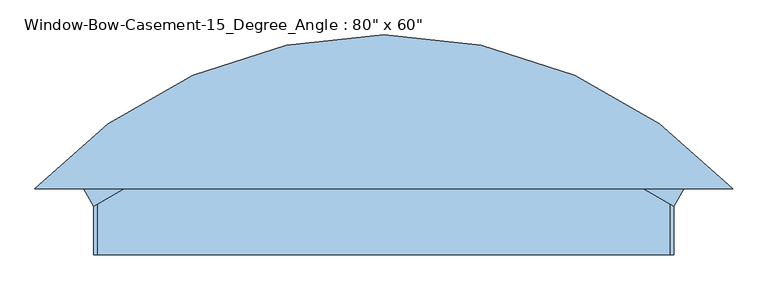
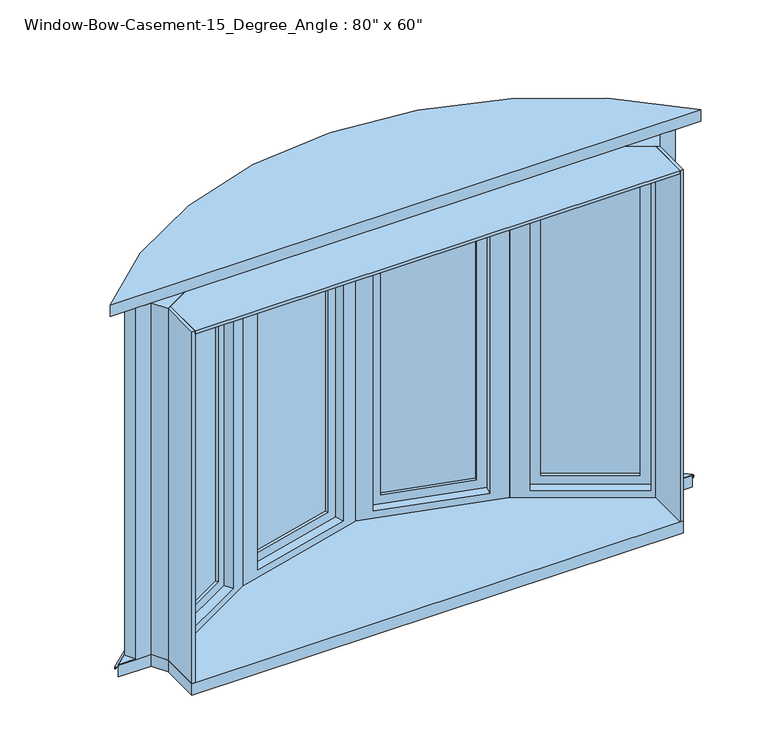
"""IFC4 building model written with IfcOpenShell, lengths in millimetres: window geometry."""

from ifc_helpers import new_model, si_unit, point, frame, frame_2d, origin, place, context, project, spatial, polyline, circle_curve, trimmed, segment, composite_curve, outline, extrude, faceted_brep, source, transform, mapped, element, save
from ifc_brep_helpers import plane_surface, cylinder_surface, revolved_surface, advanced_brep


def window_ab94cc4f(model_context):
    return source(origin(), model_context, "Body", "SolidModel", [
        extrude(outline(polyline([(456.0794789, 416.5035982), (454.4359779, 410.3699692), (114.89545, 501.3495795), (116.5389509, 507.4832084), (456.0794789, 416.5035982)])), frame((0.0, 0.0, 730.25), z_axis=(0.0, 0.0, 1.0), x_axis=(1.0, 0.0, 0.0)), (0.0, 0.0, 1.0), 1384.3),
        extrude(outline(polyline([(452.792477, 404.2363402), (451.1489761, 398.1027112), (111.6084481, 489.0823215), (113.2519491, 495.2159505), (452.792477, 404.2363402)])), frame((0.0, 0.0, 730.25), z_axis=(0.0, 0.0, 1.0), x_axis=(1.0, 0.0, 0.0)), (0.0, 0.0, 1.0), 1384.3),
        extrude(outline(polyline([(1441.45, 57.15), (1441.45, -408.6682209), (-57.15, -408.6682209), (-57.15, 57.15), (1441.45, 57.15)]), holes=[polyline([(1384.3, -351.5182208), (1384.3, 0.0), (0.0, 0.0), (0.0, -351.5182208), (1384.3, -351.5182208)])]), frame((447.8619742, 385.8354532, 730.25), z_axis=(0.25881904510252074, 0.9659258262890683, 0.0), x_axis=(0.0, 0.0, 1.0)), (0.0, 0.0, 1.0), 44.45),
        faceted_brep([(0.0, 466.395685, 2184.4), (545.6573362, 320.1872425, 2184.4), (584.8734724, 414.8633704, 2184.4), (0.0, 571.579745, 2184.4), (503.0646352, 371.0439448, 2171.7), (53.1187853, 491.6065719, 2171.7), (69.5537947, 552.9428619, 2171.7), (519.4996445, 432.3802348, 2171.7), (474.8027426, 339.1726736, 2152.65), (61.6586667, 449.8742951, 2152.65), (71.5196723, 486.6760691, 2152.65), (484.6637482, 375.9744476, 2152.65), (53.1187853, 491.6065719, 673.1), (69.5537947, 552.9428619, 673.1), (61.6586667, 449.8742951, 692.15), (71.5196723, 486.6760691, 692.15), (0.0, 571.579745, 660.4), (584.8734724, 414.8633704, 660.4), (545.6573362, 320.1872425, 660.4), (0.0, 466.395685, 660.4), (503.0646352, 371.0439448, 673.1), (519.4996445, 432.3802348, 673.1), (474.8027426, 339.1726736, 692.15), (484.6637482, 375.9744476, 692.15)], [[[0, 1, 2, 3]], [[4, 5, 6, 7]], [[8, 9, 10, 11]], [[5, 12, 13, 6]], [[9, 14, 15, 10]], [[16, 17, 18, 19]], [[12, 20, 21, 13]], [[14, 22, 23, 15]], [[2, 17, 16, 3], [6, 13, 21, 7]], [[7, 21, 20, 4]], [[4, 20, 12, 5], [10, 15, 23, 11]], [[11, 23, 22, 8]], [[18, 1, 0, 19], [8, 22, 14, 9]], [[3, 16, 19, 0]], [[1, 18, 17, 2]]]),
        extrude(outline(polyline([(-456.0794789, 416.5035982), (-116.5389509, 507.4832084), (-114.89545, 501.3495795), (-454.4359779, 410.3699692), (-456.0794789, 416.5035982)])), frame((0.0, 0.0, 730.25), z_axis=(0.0, 0.0, 1.0), x_axis=(1.0, 0.0, 0.0)), (0.0, 0.0, 1.0), 1384.3),
        extrude(outline(polyline([(-452.792477, 404.2363402), (-113.2519491, 495.2159505), (-111.6084481, 489.0823215), (-451.1489761, 398.1027112), (-452.792477, 404.2363402)])), frame((0.0, 0.0, 730.25), z_axis=(0.0, 0.0, 1.0), x_axis=(1.0, 0.0, 0.0)), (0.0, 0.0, 1.0), 1384.3),
        extrude(outline(polyline([(1441.45, -57.15), (-57.15, -57.15), (-57.15, 408.6682209), (1441.45, 408.6682209), (1441.45, -57.15)]), holes=[polyline([(1384.3, 351.5182208), (0.0, 351.5182208), (0.0, 0.0), (1384.3, 0.0), (1384.3, 351.5182208)])]), frame((-447.8619742, 385.8354532, 730.25), z_axis=(-0.25881904510252074, 0.9659258262890683, 0.0), x_axis=(0.0, 0.0, 1.0)), (0.0, 0.0, 1.0), 44.45),
        faceted_brep([(0.0, 466.395685, 2184.4), (0.0, 571.579745, 2184.4), (-584.8734724, 414.8633704, 2184.4), (-545.6573362, 320.1872425, 2184.4), (-503.0646352, 371.0439448, 2171.7), (-519.4996445, 432.3802348, 2171.7), (-69.5537947, 552.9428619, 2171.7), (-53.1187853, 491.6065719, 2171.7), (-474.8027426, 339.1726736, 2152.65), (-484.6637482, 375.9744476, 2152.65), (-71.5196723, 486.6760691, 2152.65), (-61.6586667, 449.8742951, 2152.65), (-69.5537947, 552.9428619, 673.1), (-53.1187853, 491.6065719, 673.1), (-71.5196723, 486.6760691, 692.15), (-61.6586667, 449.8742951, 692.15), (0.0, 571.579745, 660.4), (0.0, 466.395685, 660.4), (-545.6573362, 320.1872425, 660.4), (-584.8734724, 414.8633704, 660.4), (-519.4996445, 432.3802348, 673.1), (-503.0646352, 371.0439448, 673.1), (-484.6637482, 375.9744476, 692.15), (-474.8027426, 339.1726736, 692.15)], [[[0, 1, 2, 3]], [[4, 5, 6, 7]], [[8, 9, 10, 11]], [[7, 6, 12, 13]], [[11, 10, 14, 15]], [[16, 17, 18, 19]], [[13, 12, 20, 21]], [[15, 14, 22, 23]], [[2, 1, 16, 19], [6, 5, 20, 12]], [[5, 4, 21, 20]], [[4, 7, 13, 21], [10, 9, 22, 14]], [[9, 8, 23, 22]], [[18, 17, 0, 3], [8, 11, 15, 23]], [[1, 0, 17, 16]], [[3, 2, 19, 18]]]),
        extrude(outline(polyline([(981.6166025, 149.225), (978.4416025, 143.7257387), (674.0178933, 319.4848491), (677.1928933, 324.9841104), (981.6166025, 149.225)])), frame((0.0, 0.0, 730.25), z_axis=(0.0, 0.0, 1.0), x_axis=(1.0, 0.0, 0.0)), (0.0, 0.0, 1.0), 1384.3),
        extrude(outline(polyline([(975.2666025, 138.2264774), (972.0916025, 132.7272161), (667.6678933, 308.4863265), (670.8428933, 313.9855878), (975.2666025, 138.2264774)])), frame((0.0, 0.0, 730.25), z_axis=(0.0, 0.0, 1.0), x_axis=(1.0, 0.0, 0.0)), (0.0, 0.0, 1.0), 1384.3),
        extrude(outline(polyline([(1441.45, 57.15), (1441.45, -408.6682209), (-57.15, -408.6682209), (-57.15, 57.15), (1441.45, 57.15)]), holes=[polyline([(1384.3, -351.5182209), (1384.3, 0.0), (0.0, 0.0), (0.0, -351.5182209), (1384.3, -351.5182209)])]), frame((965.7416025, 121.7286934, 730.25), z_axis=(0.5, 0.8660254037844387, 0.0), x_axis=(0.0, 0.0, 1.0)), (0.0, 0.0, 1.0), 44.45),
        faceted_brep([(545.7458347, 320.2192725, 2184.4), (1007.1834769, 53.8081255, 2184.4), (1042.1084769, 114.3, 2184.4), (1105.6084769, 114.3, 2184.4), (584.9619709, 414.8954004, 2184.4), (1015.2349543, 93.1536934, 2171.7), (611.8245415, 326.0628039, 2171.7), (643.5745415, 381.055417, 2171.7), (1046.9849543, 148.1463066, 2171.7), (979.6871704, 69.6831255, 2152.65), (609.2723254, 283.542236, 2152.65), (628.3223254, 316.5378039, 2152.65), (998.7371704, 102.6786934, 2152.65), (611.8245415, 326.0628039, 673.1), (643.5745415, 381.055417, 673.1), (609.2723254, 283.542236, 692.15), (628.3223254, 316.5378039, 692.15), (584.9619709, 414.8954004, 660.4), (1105.6084769, 114.3, 660.4), (1042.1084769, 114.3, 660.4), (1007.1834769, 53.8081255, 660.4), (545.7458347, 320.2192725, 660.4), (1015.2349543, 93.1536934, 673.1), (1046.9849543, 148.1463066, 673.1), (979.6871704, 69.6831255, 692.15), (998.7371704, 102.6786934, 692.15)], [[[0, 1, 2, 3, 4]], [[5, 6, 7, 8]], [[9, 10, 11, 12]], [[6, 13, 14, 7]], [[10, 15, 16, 11]], [[17, 18, 19, 20, 21]], [[13, 22, 23, 14]], [[15, 24, 25, 16]], [[20, 19, 2, 1]], [[3, 18, 17, 4], [7, 14, 23, 8]], [[8, 23, 22, 5]], [[5, 22, 13, 6], [11, 16, 25, 12]], [[12, 25, 24, 9]], [[1, 0, 21, 20], [9, 24, 15, 10]], [[2, 19, 18, 3]], [[4, 17, 21, 0]]]),
        extrude(outline(polyline([(-981.6166025, 149.225), (-677.1928933, 324.9841104), (-674.0178933, 319.4848491), (-978.4416025, 143.7257387), (-981.6166025, 149.225)])), frame((0.0, 0.0, 730.25), z_axis=(0.0, 0.0, 1.0), x_axis=(1.0, 0.0, 0.0)), (0.0, 0.0, 1.0), 1384.3),
        extrude(outline(polyline([(-975.2666025, 138.2264774), (-670.8428933, 313.9855878), (-667.6678933, 308.4863265), (-972.0916025, 132.7272161), (-975.2666025, 138.2264774)])), frame((0.0, 0.0, 730.25), z_axis=(0.0, 0.0, 1.0), x_axis=(1.0, 0.0, 0.0)), (0.0, 0.0, 1.0), 1384.3),
        extrude(outline(polyline([(1441.45, -57.15), (-57.15, -57.15), (-57.15, 408.6682209), (1441.45, 408.6682209), (1441.45, -57.15)]), holes=[polyline([(1384.3, 351.5182209), (0.0, 351.5182209), (0.0, 0.0), (1384.3, 0.0), (1384.3, 351.5182209)])]), frame((-965.7416025, 121.7286934, 730.25), z_axis=(-0.5, 0.8660254037844387, 0.0), x_axis=(0.0, 0.0, 1.0)), (0.0, 0.0, 1.0), 44.45),
        faceted_brep([(-545.7458347, 320.2192725, 2184.4), (-584.9619709, 414.8954004, 2184.4), (-1105.6084769, 114.3, 2184.4), (-1042.1084769, 114.3, 2184.4), (-1007.1834769, 53.8081255, 2184.4), (-1015.2349543, 93.1536934, 2171.7), (-1046.9849543, 148.1463066, 2171.7), (-643.5745415, 381.055417, 2171.7), (-611.8245415, 326.0628039, 2171.7), (-979.6871704, 69.6831255, 2152.65), (-998.7371704, 102.6786934, 2152.65), (-628.3223254, 316.5378039, 2152.65), (-609.2723254, 283.542236, 2152.65), (-643.5745415, 381.055417, 673.1), (-611.8245415, 326.0628039, 673.1), (-628.3223254, 316.5378039, 692.15), (-609.2723254, 283.542236, 692.15), (-584.9619709, 414.8954004, 660.4), (-545.7458347, 320.2192725, 660.4), (-1007.1834769, 53.8081255, 660.4), (-1042.1084769, 114.3, 660.4), (-1105.6084769, 114.3, 660.4), (-1046.9849543, 148.1463066, 673.1), (-1015.2349543, 93.1536934, 673.1), (-998.7371704, 102.6786934, 692.15), (-979.6871704, 69.6831255, 692.15)], [[[0, 1, 2, 3, 4]], [[5, 6, 7, 8]], [[9, 10, 11, 12]], [[8, 7, 13, 14]], [[12, 11, 15, 16]], [[17, 18, 19, 20, 21]], [[14, 13, 22, 23]], [[16, 15, 24, 25]], [[19, 4, 3, 20]], [[2, 1, 17, 21], [7, 6, 22, 13]], [[6, 5, 23, 22]], [[5, 8, 14, 23], [11, 10, 24, 15]], [[10, 9, 25, 24]], [[4, 19, 18, 0], [9, 12, 16, 25]], [[3, 2, 21, 20]], [[1, 0, 18, 17]]]),
        advanced_brep(
        [(-1176.4506644, 114.3, 663.1486341), (-1176.4506644, 114.3, 660.4), (-1105.6250672, 114.3, 660.4), (-1105.6250672, 114.3, 663.1486341), (1176.4506644, 114.3, 660.4), (1176.4506644, 114.3, 663.1486341), (1105.6250672, 114.3, 663.1486341), (1105.6250672, 114.3, 660.4), (-1176.4506644, 114.3, 653.0697935), (-1177.4675315, 115.2579093, 663.1486341), (-1177.4675315, 115.2579093, 654.4483503), (-1186.7117777, 123.9661762, 652.2089977), (-1186.7117777, 123.9661762, 643.2668038), (-1183.8275729, 121.249197, 643.2668038), (-1183.8275729, 121.249197, 644.7270038), (-1185.5470027, 122.8689346, 644.7270038), (-1185.5470027, 122.8689346, 650.8662705), (1176.4506644, 114.3, 653.0697935), (1185.5470027, 122.8689346, 650.8662705), (1185.5470027, 122.8689346, 644.7270038), (1183.8275729, 121.249197, 644.7270038), (1183.8275729, 121.249197, 643.2668038), (1186.7117777, 123.9661762, 643.2668038), (1186.7117777, 123.9661762, 652.2089977), (1177.4675315, 115.2579093, 654.4483503), (1177.4675315, 115.2579093, 663.1486341)],
        [
            (0, 1),
            (1, 2),
            (2, 3),
            (3, 0),
            (4, 5),
            (5, 6),
            (6, 7),
            (7, 4),
            (8, 1),
            (0, 9),
            (9, 10),
            (10, 11),
            (11, 12),
            (12, 13),
            (13, 14),
            (14, 15),
            (15, 16),
            (16, 8),
            (17, 18),
            (18, 19),
            (19, 20),
            (20, 21),
            (21, 22),
            (22, 23),
            (23, 24),
            (24, 25),
            (25, 5),
            (4, 17),
            (8, 17, circle_curve(frame((0.0, -993.9403207, 653.0697935), z_axis=(0.0, 0.0, -1.0), x_axis=(-0.7278934013453495, 0.6856903063905001, 0.0)), 1616.2403207)),
            (4, 1, circle_curve(frame((0.0, -993.9403207, 660.4), z_axis=(0.0, 0.0, 1.0), x_axis=(-0.7278934013453495, 0.6856903063905001, 0.0)), 1616.2403207)),
            (7, 2, circle_curve(frame((0.0, -993.9403207, 660.4), z_axis=(0.0, 0.0, 1.0), x_axis=(-0.7278934013453495, 0.6856903063905001, 0.0)), 1565.4403207)),
            (6, 3, circle_curve(frame((0.0, -993.9403207, 663.1486341), z_axis=(0.0, 0.0, 1.0), x_axis=(-0.7278934013453495, 0.6856903063905001, 0.0)), 1565.4403207)),
            (25, 9, circle_curve(frame((0.0, -993.9403207, 663.1486341), z_axis=(0.0, 0.0, 1.0), x_axis=(-0.7278934013453495, 0.6856903063905001, 0.0)), 1617.6373207)),
            (24, 10, circle_curve(frame((0.0, -993.9403207, 654.4483503), z_axis=(0.0, 0.0, 1.0), x_axis=(-0.7278934013453495, 0.6856903063905001, 0.0)), 1617.6373207)),
            (23, 11, circle_curve(frame((0.0, -993.9403207, 652.2089977), z_axis=(0.0, 0.0, 1.0), x_axis=(-0.7278934013453495, 0.6856903063905001, 0.0)), 1630.3373207)),
            (22, 12, circle_curve(frame((0.0, -993.9403207, 643.2668038), z_axis=(0.0, 0.0, 1.0), x_axis=(-0.7278934013453495, 0.6856903063905001, 0.0)), 1630.3373207)),
            (21, 13, circle_curve(frame((0.0, -993.9403207, 643.2668038), z_axis=(0.0, 0.0, 1.0), x_axis=(-0.7278934013453495, 0.6856903063905001, 0.0)), 1626.3749208)),
            (20, 14, circle_curve(frame((0.0, -993.9403207, 644.7270038), z_axis=(0.0, 0.0, 1.0), x_axis=(-0.7278934013453495, 0.6856903063905001, 0.0)), 1626.3749208)),
            (19, 15, circle_curve(frame((0.0, -993.9403207, 644.7270038), z_axis=(0.0, 0.0, 1.0), x_axis=(-0.7278934013453495, 0.6856903063905001, 0.0)), 1628.7371207)),
            (18, 16, circle_curve(frame((0.0, -993.9403207, 650.8662705), z_axis=(0.0, 0.0, 1.0), x_axis=(-0.7278934013453495, 0.6856903063905001, 0.0)), 1628.7371207)),
        ],
        [
            plane_surface(frame((1259.3975394, 114.3, 1270.0), z_axis=(0.0, -1.0, 0.0), x_axis=(0.0, 0.0, -1.0))),
            plane_surface(frame((-1176.4506644, 114.3, 660.4), z_axis=(-0.6856903063905001, -0.7278934013453495, 0.0), x_axis=(0.0, 0.0, 1.0))),
            plane_surface(frame((1176.4506644, 114.3, 660.4), z_axis=(0.6856903063904999, -0.7278934013453497, 0.0), x_axis=(0.0, 0.0, 1.0))),
            revolved_surface(polyline([(-1176.4506644258215, 114.3000000014631, 653.0697935), (-1176.4506644258215, 114.3000000014631, 660.4)]), (0.0, -993.9403207, 660.4), (0.0, 0.0, -1.0)),
            plane_surface(frame((0.0, -993.9403207, 660.4), z_axis=(0.0, 0.0, -1.0), x_axis=(-0.7278934013453495, 0.6856903063905001, 0.0))),
            revolved_surface(polyline([(-1139.4736796374777, 79.4669324368258, 660.4), (-1139.4736796374777, 79.4669324368258, 663.1486341)]), (0.0, -993.9403207, 660.4), (0.0, 0.0, -1.0)),
            plane_surface(frame((0.0, -993.9403207, 663.1486341), z_axis=(0.0, 0.0, 1.0), x_axis=(-0.7278934013453495, 0.6856903063905001, 0.0))),
            cylinder_surface(frame((0.0, -993.9403207, 660.4), z_axis=(0.0, 0.0, -1.0), x_axis=(-0.7278934013453495, 0.6856903063905001, 0.0)), 1617.6373207),
            revolved_surface(polyline([(-1177.4675315, 115.2579093, 654.4483503), (-1186.7117777, 123.9661762, 652.2089977)]), (0.0, -993.9403207, 660.4), (0.0, 0.0, -1.0)),
            cylinder_surface(frame((0.0, -993.9403207, 660.4), z_axis=(0.0, 0.0, -1.0), x_axis=(-0.7278934013453495, 0.6856903063905001, 0.0)), 1630.3373207),
            plane_surface(frame((0.0, -993.9403207, 643.2668038), z_axis=(0.0, 0.0, -1.0), x_axis=(-0.7278934013453495, 0.6856903063905001, 0.0))),
            revolved_surface(polyline([(-1183.8275729638854, 121.24919704917716, 643.2668038), (-1183.8275729638854, 121.24919704917716, 644.7270038)]), (0.0, -993.9403207, 660.4), (0.0, 0.0, -1.0)),
            plane_surface(frame((0.0, -993.9403207, 644.7270038), z_axis=(0.0, 0.0, 1.0), x_axis=(-0.7278934013453495, 0.6856903063905001, 0.0))),
            revolved_surface(polyline([(-1185.5470026837543, 122.8689346223639, 644.7270038), (-1185.5470026837543, 122.8689346223639, 650.8662705)]), (0.0, -993.9403207, 660.4), (0.0, 0.0, -1.0)),
            revolved_surface(polyline([(-1185.5470027, 122.8689346, 650.8662705), (-1176.4506644, 114.3, 653.0697935)]), (0.0, -993.9403207, 660.4), (0.0, 0.0, -1.0)),
        ],
        [
            (0, [[1, 2, 3, 4]]),
            (0, [[5, 6, 7, 8]]),
            (1, [[9, -1, 10, 11, 12, 13, 14, 15, 16, 17, 18]]),
            (2, [[19, 20, 21, 22, 23, 24, 25, 26, 27, -5, 28]]),
            (3, [[-9, 29, -28, 30]]),
            (4, [[-30, -8, 31, -2]]),
            (5, [[-31, -7, 32, -3]]),
            (6, [[33, -10, -4, -32, -6, -27]]),
            (7, [[-11, -33, -26, 34]]),
            (8, [[-12, -34, -25, 35]]),
            (9, [[-13, -35, -24, 36]]),
            (10, [[-14, -36, -23, 37]]),
            (11, [[-15, -37, -22, 38]]),
            (12, [[-16, -38, -21, 39]]),
            (13, [[-17, -39, -20, 40]]),
            (14, [[-18, -40, -19, -29]]),
        ],
    ),
        extrude(outline(polyline([(-1078.1121704, 130.175), (-1105.6084769, 114.3), (-1127.8334769, 152.7948292), (-1100.3371704, 168.6698292), (-1078.1121704, 130.175)])), frame((0.0, 0.0, 663.1486341), z_axis=(0.0, 0.0, 1.0), x_axis=(1.0, 0.0, 0.0)), (0.0, 0.0, 1.0), 1521.2513659),
        extrude(outline(polyline([(1078.1121704, 130.175), (1100.3371704, 168.6698292), (1127.8334769, 152.7948292), (1105.6084769, 114.3), (1078.1121704, 130.175)])), frame((0.0, 0.0, 663.1486341), z_axis=(0.0, 0.0, 1.0), x_axis=(1.0, 0.0, 0.0)), (0.0, 0.0, 1.0), 1521.2513659),
        extrude(outline(composite_curve([segment(trimmed(circle_curve(frame_2d((0.0, -993.9568727)), 1641.6403207), [point((-1211.0944004, 114.3))], [point((1211.0944004, 114.3))], False, "CARTESIAN"), True, "CONTINUOUS"), segment(polyline([(1211.0944004, 114.3), (-1211.0944004, 114.3)]), True, "CONTINUOUS")], self_intersect=False)), frame((0.0, 0.0, 2184.4), z_axis=(0.0, 0.0, 1.0), x_axis=(1.0, 0.0, 0.0)), (0.0, 0.0, 1.0), 50.8),
        extrude(outline(composite_curve([segment(polyline([(1007.1834769, -114.3), (-1007.1834769, -114.3), (-1007.1834769, 53.8081255), (-1042.1084769, 114.3), (-1176.4249956, 114.3)]), True, "CONTINUOUS"), segment(trimmed(circle_curve(frame_2d((0.0, -993.9675688)), 1616.2403207), [point((-1176.4249956, 114.3))], [point((1176.4249956, 114.3))], False, "CARTESIAN"), True, "CONTINUOUS"), segment(polyline([(1176.4249956, 114.3), (1042.1084769, 114.3), (1007.1834769, 53.8081255), (1007.1834769, -114.3)]), True, "CONTINUOUS")], self_intersect=False)), frame((0.0, 0.0, 609.6), z_axis=(0.0, 0.0, 1.0), x_axis=(1.0, 0.0, 0.0)), (0.0, 0.0, 1.0), 50.8),
        extrude(outline(polyline([(-1007.1834769, -114.3), (-1007.1834769, 53.8081255), (-994.4834769, 61.140474), (-994.4834769, -114.3), (-1007.1834769, -114.3)])), frame((0.0, 0.0, 660.4), z_axis=(0.0, 0.0, 1.0), x_axis=(1.0, 0.0, 0.0)), (0.0, 0.0, 1.0), 1524.0),
        extrude(outline(polyline([(1007.1834769, -114.3), (994.4834769, -114.3), (994.4834769, 61.140474), (1007.1834769, 53.8081255), (1007.1834769, -114.3)])), frame((0.0, 0.0, 660.4), z_axis=(0.0, 0.0, 1.0), x_axis=(1.0, 0.0, 0.0)), (0.0, 0.0, 1.0), 1524.0),
        extrude(outline(polyline([(-545.7458347, 320.2192725), (0.0, 466.4514281), (545.7458347, 320.2192725), (994.4834769, 61.140474), (994.4834769, -114.3), (-994.4834769, -114.3), (-994.4834769, 61.140474), (-545.7458347, 320.2192725)])), frame((0.0, 0.0, 2171.7), z_axis=(0.0, 0.0, 1.0), x_axis=(1.0, 0.0, 0.0)), (0.0, 0.0, 1.0), 12.7),
    ])


if __name__ == "__main__":
    model = new_model("IFC4")
    model_context = context("Model", 3, world=origin())
    ifc_project = project(units=[si_unit("LENGTHUNIT", "METRE", prefix="MILLI")], contexts=[model_context])
    site = spatial("IfcSite", under=ifc_project)
    building = spatial("IfcBuilding", under=site)
    placement = place(None, origin())
    window_shape = window_ab94cc4f(model_context)
    element("IfcWindow", 1, ObjectType="Window-Bow-Casement-15_Degree_Angle : 80\" x 60\"", at=placement, inside=building, context=model_context, shape_type="MappedRepresentation", body=[
        mapped(window_shape, transform((0.0, 0.0, 0.0), x_axis=(1.0, 0.0, 0.0), y_axis=(0.0, 1.0, 0.0), z_axis=(0.0, 0.0, 1.0))),
    ])
    save(model, "model.ifc")

# Revit data of these elements
# Type "Window-Bow-Casement-15_Degree_Angle : 80\" x 60\""
#   Type Mark = "19"
#   Fire Rating = "0.5h"
#   Assembly Code = "B2020100"
#   Analytic Construction = "Double glazing - domestic"
#   Width = 6' - 7.30579"
#   Visual Light Transmittance = 0.81
#   Thermal Resistance (R) = 1.8146 (h·ft²·°F)/BTU
#   Solar Heat Gain Coefficient = 0.76
#   Rough Width = 6' - 7.80579"
#   Rough Height = 5' - 0 1/2"
#   Length 3 = 0' - 1 239/256"
#   Height 1 = 5' - 2"
#   Height = 5' - 0"
#   Heat Transfer Coefficient (U) = 0.5511 BTU/(h·ft²·°F)
#   Depth 7 = 0' - 0 83/128"
#   Depth 6 = 0' - 1 207/256"
#   Depth 5 = 0' - 2.16481"
#   Depth 4 = 0' - 1.16481"
#   Width of Middle Sash = 3' - 5.22785"
#   Radius 2 = 5' - 4.63151"
#   Radius 1 = 5' - 3.63151"
#   Length 2 = 7' - 3.05579"
#   Length 1 = 1' - 5.10538"
#   Wall Thickness [instance default] = 0' - 6"
#   Trim Width = 6' - 11.97766"
#   Depth 3 = 0' - 5.00538"
#   Depth 2 = 0' - 6.16554"
#   Depth 1 = 0' - 11.83446"
#   Depth = 1' - 6"
#   Default Sill Height = 2' - 0"
#   Angle 2 = 15.00°
#   Angle 1 = 30.00°
#   Muntin Visibility = yes
#   Interior Trim Visibility [instance default] = yes
#   Exterior Trim Visibility [instance default] = yes
#   Interior Trim Material = Wood - Stained
#   Exterior Trim Material = Clad - White
#   Muntin Pattern = Muntin Pattern_2x2 : Muntin Pattern_2x2
#   Exterior Trim = element 398010
#   Interior Trim = Trim-Window-Interior-Flat : Picture Frame
#   Interior Frame Material = Wood - Stained
#   Glass Panel Material = Glass
#   Exterior Frame Material = Clad - White
#   Wall Closure = (empty or 0)
# Element 1 (IfcWindow, "Window-Bow-Casement-15_Degree_Angle : 80\" x 60\"")
#   Wall Thickness = 0' - 9"
#   Materials on its faces: "Wood - Stained", "Clad - White", "Glass"
# Materials
#   "Wood - Stained": class "Wood", colour RGB 224 178 126, transparency 0, Cost = 0
#   "Clad - White": class "Wood", colour RGB 242 242 238, transparency 0, Cost = 0
#   "Glass": class "Glass", colour RGB 0 128 192, transparency 0.75, Description = "Soda Lime Glass", Cost = 0
